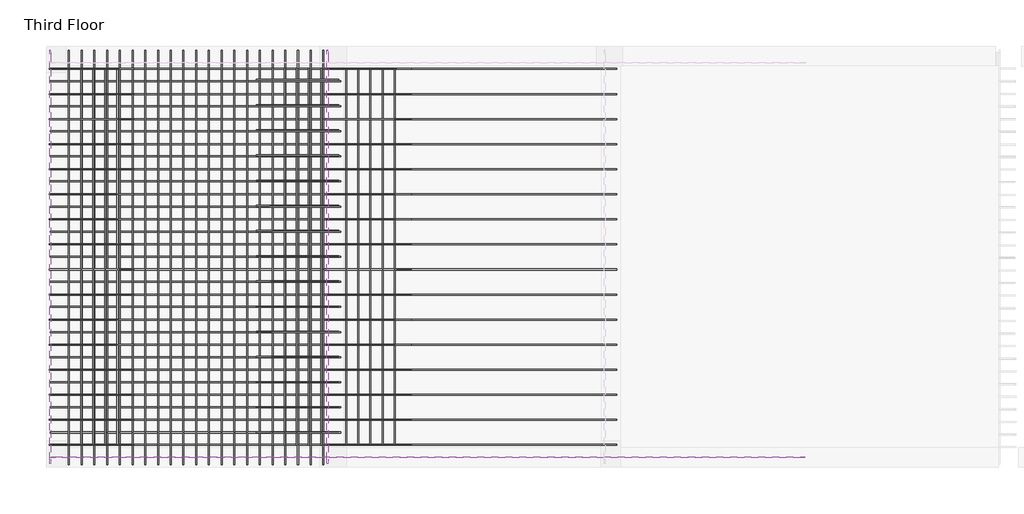
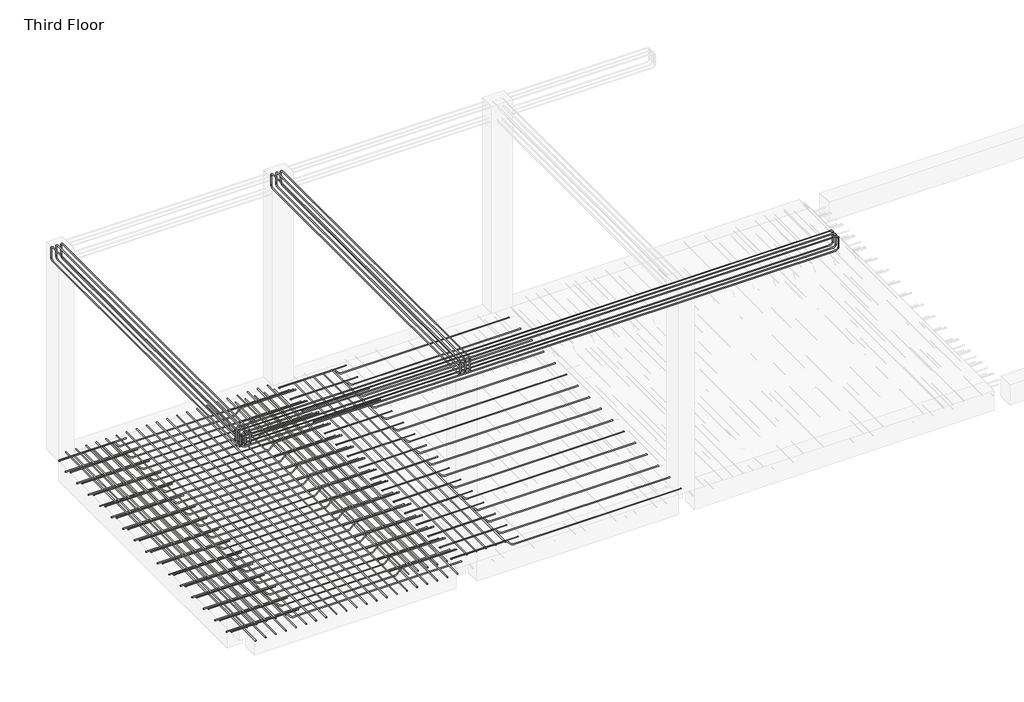
# One storey, part 2 of 4: 16 reinforcing bars.
"""IFC4 building model written with IfcOpenShell, lengths in millimetres."""

from ifc_helpers import new_model, si_unit, point, frame, origin, place, context, project, spatial, polyline, circle_curve, trimmed, segment, composite_curve, source, transform, mapped, element, save
from ifc_brep_helpers import swept_disk

model = new_model("IFC4")

# Units and contexts
model_context = context("Model", 3, world=origin())
ifc_project = project(units=[si_unit("LENGTHUNIT", "METRE", prefix="MILLI")], contexts=[model_context])

# Site, building, storey
site = spatial("IfcSite", under=ifc_project)
building = spatial("IfcBuilding", under=site)
storey = spatial("IfcBuildingStorey", under=building, Name="Third Floor", Elevation=9601.2)

# Reinforcing bars
placement = place(None, origin())
reinforcing_bar_shape = source(origin(), model_context, "Body", "SolidModel", [
    swept_disk(composite_curve([segment(polyline([(-9335.8112474, 5017.2334631, 12564.4994949), (-9335.8112474, 5017.2334631, 12712.4994949)]), True, "CONTINUOUS"), segment(trimmed(circle_curve(frame((-9335.8112474, 4971.2334631, 12712.4994949), z_axis=(1.0, 0.0, 0.0), x_axis=(0.0, 46.0, 0.0)), 46.0), [point((-9335.8112474, 5017.2334631, 12712.4994949))], [point((-9335.8112474, 4971.2334631, 12758.4994949))], True, "CARTESIAN"), True, "CONTINUOUS"), segment(polyline([(-9335.8112474, 4971.2334631, 12758.4994949), (-9335.8112474, 278.4334631, 12758.4994949)]), True, "CONTINUOUS"), segment(trimmed(circle_curve(frame((-9335.8112474, 278.4334631, 12712.4994949), z_axis=(1.0, 0.0, 0.0), x_axis=(0.0, 0.0, 46.0)), 46.0), [point((-9335.8112474, 278.4334631, 12758.4994949))], [point((-9335.8112474, 232.4334631, 12712.4994949))], True, "CARTESIAN"), True, "CONTINUOUS"), segment(polyline([(-9335.8112474, 232.4334631, 12712.4994949), (-9335.8112474, 232.4334631, 12564.4994949)]), True, "CONTINUOUS")], self_intersect=False), 6.0),
])
element("IfcReinforcingBar", 1, at=placement, inside=storey, context=model_context, shape_type="MappedRepresentation", body=[
    mapped(reinforcing_bar_shape, transform((0.0, 0.0, 0.0), x_axis=(1.0, 0.0, 0.0), y_axis=(0.0, 1.0, 0.0), z_axis=(0.0, 0.0, 1.0))),
    mapped(reinforcing_bar_shape, transform((71.1994949, 0.0, 0.0), x_axis=(1.0, 0.0, 0.0), y_axis=(0.0, 1.0, 0.0), z_axis=(0.0, 0.0, 1.0))),
    mapped(reinforcing_bar_shape, transform((142.3989899, 0.0, 0.0), x_axis=(1.0, 0.0, 0.0), y_axis=(0.0, 1.0, 0.0), z_axis=(0.0, 0.0, 1.0))),
])
reinforcing_bar_2_shape = source(origin(), model_context, "Body", "SolidModel", [
    swept_disk(composite_curve([segment(polyline([(-9335.8112474, 5017.2334631, 12733.9005051), (-9335.8112474, 5017.2334631, 12585.9005051)]), True, "CONTINUOUS"), segment(trimmed(circle_curve(frame((-9335.8112474, 4971.2334631, 12585.9005051), z_axis=(-1.0, 0.0, 0.0), x_axis=(0.0, 46.0, 0.0)), 46.0), [point((-9335.8112474, 5017.2334631, 12585.9005051))], [point((-9335.8112474, 4971.2334631, 12539.9005051))], True, "CARTESIAN"), True, "CONTINUOUS"), segment(polyline([(-9335.8112474, 4971.2334631, 12539.9005051), (-9335.8112474, 278.4334631, 12539.9005051)]), True, "CONTINUOUS"), segment(trimmed(circle_curve(frame((-9335.8112474, 278.4334631, 12585.9005051), z_axis=(-1.0, 0.0, 0.0), x_axis=(0.0, 0.0, -46.0)), 46.0), [point((-9335.8112474, 278.4334631, 12539.9005051))], [point((-9335.8112474, 232.4334631, 12585.9005051))], True, "CARTESIAN"), True, "CONTINUOUS"), segment(polyline([(-9335.8112474, 232.4334631, 12585.9005051), (-9335.8112474, 232.4334631, 12733.9005051)]), True, "CONTINUOUS")], self_intersect=False), 6.0),
])
element("IfcReinforcingBar", 2, at=placement, inside=storey, context=model_context, shape_type="MappedRepresentation", body=[
    mapped(reinforcing_bar_2_shape, transform((0.0, 0.0, 0.0), x_axis=(1.0, 0.0, 0.0), y_axis=(0.0, 1.0, 0.0), z_axis=(0.0, 0.0, 1.0))),
    mapped(reinforcing_bar_2_shape, transform((71.1994949, 0.0, 0.0), x_axis=(1.0, 0.0, 0.0), y_axis=(0.0, 1.0, 0.0), z_axis=(0.0, 0.0, 1.0))),
    mapped(reinforcing_bar_2_shape, transform((142.3989899, 0.0, 0.0), x_axis=(1.0, 0.0, 0.0), y_axis=(0.0, 1.0, 0.0), z_axis=(0.0, 0.0, 1.0))),
])
reinforcing_bar_3_shape = source(origin(), model_context, "Body", "SolidModel", [
    swept_disk(composite_curve([segment(polyline([(-6122.7112474, 5017.2334631, 12564.4994949), (-6122.7112474, 5017.2334631, 12712.4994949)]), True, "CONTINUOUS"), segment(trimmed(circle_curve(frame((-6122.7112474, 4971.2334631, 12712.4994949), z_axis=(1.0, 0.0, 0.0), x_axis=(0.0, 46.0, 0.0)), 46.0), [point((-6122.7112474, 5017.2334631, 12712.4994949))], [point((-6122.7112474, 4971.2334631, 12758.4994949))], True, "CARTESIAN"), True, "CONTINUOUS"), segment(polyline([(-6122.7112474, 4971.2334631, 12758.4994949), (-6122.7112474, 278.4334631, 12758.4994949)]), True, "CONTINUOUS"), segment(trimmed(circle_curve(frame((-6122.7112474, 278.4334631, 12712.4994949), z_axis=(1.0, 0.0, 0.0), x_axis=(0.0, 0.0, 46.0)), 46.0), [point((-6122.7112474, 278.4334631, 12758.4994949))], [point((-6122.7112474, 232.4334631, 12712.4994949))], True, "CARTESIAN"), True, "CONTINUOUS"), segment(polyline([(-6122.7112474, 232.4334631, 12712.4994949), (-6122.7112474, 232.4334631, 12564.4994949)]), True, "CONTINUOUS")], self_intersect=False), 6.0),
])
element("IfcReinforcingBar", 3, at=placement, inside=storey, context=model_context, shape_type="MappedRepresentation", body=[
    mapped(reinforcing_bar_3_shape, transform((0.0, 0.0, 0.0), x_axis=(1.0, 0.0, 0.0), y_axis=(0.0, 1.0, 0.0), z_axis=(0.0, 0.0, 1.0))),
    mapped(reinforcing_bar_3_shape, transform((71.1994949, 0.0, 0.0), x_axis=(1.0, 0.0, 0.0), y_axis=(0.0, 1.0, 0.0), z_axis=(0.0, 0.0, 1.0))),
    mapped(reinforcing_bar_3_shape, transform((142.3989899, 0.0, 0.0), x_axis=(1.0, 0.0, 0.0), y_axis=(0.0, 1.0, 0.0), z_axis=(0.0, 0.0, 1.0))),
])
reinforcing_bar_4_shape = source(origin(), model_context, "Body", "SolidModel", [
    swept_disk(composite_curve([segment(polyline([(-6122.7112474, 5017.2334631, 12733.9005051), (-6122.7112474, 5017.2334631, 12585.9005051)]), True, "CONTINUOUS"), segment(trimmed(circle_curve(frame((-6122.7112474, 4971.2334631, 12585.9005051), z_axis=(-1.0, 0.0, 0.0), x_axis=(0.0, 46.0, 0.0)), 46.0), [point((-6122.7112474, 5017.2334631, 12585.9005051))], [point((-6122.7112474, 4971.2334631, 12539.9005051))], True, "CARTESIAN"), True, "CONTINUOUS"), segment(polyline([(-6122.7112474, 4971.2334631, 12539.9005051), (-6122.7112474, 278.4334631, 12539.9005051)]), True, "CONTINUOUS"), segment(trimmed(circle_curve(frame((-6122.7112474, 278.4334631, 12585.9005051), z_axis=(-1.0, 0.0, 0.0), x_axis=(0.0, 0.0, -46.0)), 46.0), [point((-6122.7112474, 278.4334631, 12539.9005051))], [point((-6122.7112474, 232.4334631, 12585.9005051))], True, "CARTESIAN"), True, "CONTINUOUS"), segment(polyline([(-6122.7112474, 232.4334631, 12585.9005051), (-6122.7112474, 232.4334631, 12733.9005051)]), True, "CONTINUOUS")], self_intersect=False), 6.0),
])
element("IfcReinforcingBar", 4, at=placement, inside=storey, context=model_context, shape_type="MappedRepresentation", body=[
    mapped(reinforcing_bar_4_shape, transform((0.0, 0.0, 0.0), x_axis=(1.0, 0.0, 0.0), y_axis=(0.0, 1.0, 0.0), z_axis=(0.0, 0.0, 1.0))),
    mapped(reinforcing_bar_4_shape, transform((71.1994949, 0.0, 0.0), x_axis=(1.0, 0.0, 0.0), y_axis=(0.0, 1.0, 0.0), z_axis=(0.0, 0.0, 1.0))),
    mapped(reinforcing_bar_4_shape, transform((142.3989899, 0.0, 0.0), x_axis=(1.0, 0.0, 0.0), y_axis=(0.0, 1.0, 0.0), z_axis=(0.0, 0.0, 1.0))),
])
reinforcing_bar_5_shape = source(origin(), model_context, "Body", "SolidModel", [
    swept_disk(composite_curve([segment(polyline([(-9323.7564088, 229.5339681, 12564.4994949), (-9323.7564088, 229.5339681, 12712.4994949)]), True, "CONTINUOUS"), segment(trimmed(circle_curve(frame((-9277.7564088, 229.5339681, 12712.4994949), z_axis=(0.0, 1.0, 0.0), x_axis=(-46.0, 0.0, 0.0)), 46.0), [point((-9323.7564088, 229.5339681, 12712.4994949))], [point((-9277.7564088, 229.5339681, 12758.4994949))], True, "CARTESIAN"), True, "CONTINUOUS"), segment(polyline([(-9277.7564088, 229.5339681, 12758.4994949), (-642.1117524, 229.5339681, 12758.4994949)]), True, "CONTINUOUS"), segment(trimmed(circle_curve(frame((-642.1117524, 229.5339681, 12712.4994949), z_axis=(0.0, 1.0, 0.0), x_axis=(0.0, 0.0, 46.0)), 46.0), [point((-642.1117524, 229.5339681, 12758.4994949))], [point((-596.1117524, 229.5339681, 12712.4994949))], True, "CARTESIAN"), True, "CONTINUOUS"), segment(polyline([(-596.1117524, 229.5339681, 12712.4994949), (-596.1117524, 229.5339681, 12564.4994949)]), True, "CONTINUOUS")], self_intersect=False), 6.0),
])
element("IfcReinforcingBar", 5, at=placement, inside=storey, context=model_context, shape_type="MappedRepresentation", body=[
    mapped(reinforcing_bar_5_shape, transform((0.0, 0.0, 0.0), x_axis=(1.0, 0.0, 0.0), y_axis=(0.0, 1.0, 0.0), z_axis=(0.0, 0.0, 1.0))),
    mapped(reinforcing_bar_5_shape, transform((0.0, 71.1994949, 0.0), x_axis=(1.0, 0.0, 0.0), y_axis=(0.0, 1.0, 0.0), z_axis=(0.0, 0.0, 1.0))),
    mapped(reinforcing_bar_5_shape, transform((0.0, 142.3989899, 0.0), x_axis=(1.0, 0.0, 0.0), y_axis=(0.0, 1.0, 0.0), z_axis=(0.0, 0.0, 1.0))),
])
reinforcing_bar_6_shape = source(origin(), model_context, "Body", "SolidModel", [
    swept_disk(composite_curve([segment(polyline([(-9317.575971, 229.5339681, 12733.9005051), (-9317.575971, 229.5339681, 12585.9005051)]), True, "CONTINUOUS"), segment(trimmed(circle_curve(frame((-9271.575971, 229.5339681, 12585.9005051), z_axis=(0.0, -1.0, 0.0), x_axis=(-46.0, 0.0, 0.0)), 46.0), [point((-9317.575971, 229.5339681, 12585.9005051))], [point((-9271.575971, 229.5339681, 12539.9005051))], True, "CARTESIAN"), True, "CONTINUOUS"), segment(polyline([(-9271.575971, 229.5339681, 12539.9005051), (-642.1117524, 229.5339681, 12539.9005051)]), True, "CONTINUOUS"), segment(trimmed(circle_curve(frame((-642.1117524, 229.5339681, 12585.9005051), z_axis=(0.0, -1.0, 0.0), x_axis=(0.0, 0.0, -46.0)), 46.0), [point((-642.1117524, 229.5339681, 12539.9005051))], [point((-596.1117524, 229.5339681, 12585.9005051))], True, "CARTESIAN"), True, "CONTINUOUS"), segment(polyline([(-596.1117524, 229.5339681, 12585.9005051), (-596.1117524, 229.5339681, 12733.9005051)]), True, "CONTINUOUS")], self_intersect=False), 6.0),
])
element("IfcReinforcingBar", 6, at=placement, inside=storey, context=model_context, shape_type="MappedRepresentation", body=[
    mapped(reinforcing_bar_6_shape, transform((0.0, 0.0, 0.0), x_axis=(1.0, 0.0, 0.0), y_axis=(0.0, 1.0, 0.0), z_axis=(0.0, 0.0, 1.0))),
    mapped(reinforcing_bar_6_shape, transform((0.0, 71.1994949, 0.0), x_axis=(1.0, 0.0, 0.0), y_axis=(0.0, 1.0, 0.0), z_axis=(0.0, 0.0, 1.0))),
    mapped(reinforcing_bar_6_shape, transform((0.0, 142.3989899, 0.0), x_axis=(1.0, 0.0, 0.0), y_axis=(0.0, 1.0, 0.0), z_axis=(0.0, 0.0, 1.0))),
])
reinforcing_bar_7_shape = source(origin(), model_context, "Body", "SolidModel", [
    swept_disk(composite_curve([segment(polyline([(-9347.5125695, 4803.6334631, 9570.2), (-8565.5792829, 4803.6334631, 9570.2)]), True, "CONTINUOUS"), segment(trimmed(circle_curve(frame((-8565.5792829, 4803.6334631, 9524.2), z_axis=(0.0, 1.0, 0.0), x_axis=(0.0, 0.0, 46.0)), 46.0), [point((-8565.5792829, 4803.6334631, 9570.2))], [point((-8533.052371, 4803.6334631, 9556.7269119))], True, "CARTESIAN"), True, "CONTINUOUS"), segment(polyline([(-8533.052371, 4803.6334631, 9556.7269119), (-8469.5985471, 4803.6334631, 9493.2730881)]), True, "CONTINUOUS"), segment(trimmed(circle_curve(frame((-8437.0716352, 4803.6334631, 9525.8), z_axis=(0.0, -1.0000000000000002, 0.0), x_axis=(-32.526911900000414, 0.0, -32.526911899998595)), 46.0), [point((-8469.5985471, 4803.6334631, 9493.2730881))], [point((-8437.0716352, 4803.6334631, 9479.8))], True, "CARTESIAN"), True, "CONTINUOUS"), segment(polyline([(-8437.0716352, 4803.6334631, 9479.8), (-5982.0597449, 4803.6334631, 9479.8)]), True, "CONTINUOUS")], self_intersect=False), 6.0),
])
element("IfcReinforcingBar", 7, at=placement, inside=storey, context=model_context, shape_type="MappedRepresentation", body=[
    mapped(reinforcing_bar_7_shape, transform((0.0, 0.0, 0.0), x_axis=(1.0, 0.0, 0.0), y_axis=(0.0, 1.0, 0.0), z_axis=(0.0, 0.0, 1.0))),
    mapped(reinforcing_bar_7_shape, transform((0.0, -290.5066667, 0.0), x_axis=(1.0, 0.0, 0.0), y_axis=(0.0, 1.0, 0.0), z_axis=(0.0, 0.0, 1.0))),
    mapped(reinforcing_bar_7_shape, transform((0.0, -581.0133333, 0.0), x_axis=(1.0, 0.0, 0.0), y_axis=(0.0, 1.0, 0.0), z_axis=(0.0, 0.0, 1.0))),
    mapped(reinforcing_bar_7_shape, transform((0.0, -871.52, 0.0), x_axis=(1.0, 0.0, 0.0), y_axis=(0.0, 1.0, 0.0), z_axis=(0.0, 0.0, 1.0))),
    mapped(reinforcing_bar_7_shape, transform((0.0, -1162.0266667, 0.0), x_axis=(1.0, 0.0, 0.0), y_axis=(0.0, 1.0, 0.0), z_axis=(0.0, 0.0, 1.0))),
    mapped(reinforcing_bar_7_shape, transform((0.0, -1452.5333333, 0.0), x_axis=(1.0, 0.0, 0.0), y_axis=(0.0, 1.0, 0.0), z_axis=(0.0, 0.0, 1.0))),
    mapped(reinforcing_bar_7_shape, transform((0.0, -1743.04, 0.0), x_axis=(1.0, 0.0, 0.0), y_axis=(0.0, 1.0, 0.0), z_axis=(0.0, 0.0, 1.0))),
    mapped(reinforcing_bar_7_shape, transform((0.0, -2033.5466667, 0.0), x_axis=(1.0, 0.0, 0.0), y_axis=(0.0, 1.0, 0.0), z_axis=(0.0, 0.0, 1.0))),
    mapped(reinforcing_bar_7_shape, transform((0.0, -2324.0533333, 0.0), x_axis=(1.0, 0.0, 0.0), y_axis=(0.0, 1.0, 0.0), z_axis=(0.0, 0.0, 1.0))),
    mapped(reinforcing_bar_7_shape, transform((0.0, -2614.56, 0.0), x_axis=(1.0, 0.0, 0.0), y_axis=(0.0, 1.0, 0.0), z_axis=(0.0, 0.0, 1.0))),
    mapped(reinforcing_bar_7_shape, transform((0.0, -2905.0666667, 0.0), x_axis=(1.0, 0.0, 0.0), y_axis=(0.0, 1.0, 0.0), z_axis=(0.0, 0.0, 1.0))),
    mapped(reinforcing_bar_7_shape, transform((0.0, -3195.5733333, 0.0), x_axis=(1.0, 0.0, 0.0), y_axis=(0.0, 1.0, 0.0), z_axis=(0.0, 0.0, 1.0))),
    mapped(reinforcing_bar_7_shape, transform((0.0, -3486.08, 0.0), x_axis=(1.0, 0.0, 0.0), y_axis=(0.0, 1.0, 0.0), z_axis=(0.0, 0.0, 1.0))),
    mapped(reinforcing_bar_7_shape, transform((0.0, -3776.5866667, 0.0), x_axis=(1.0, 0.0, 0.0), y_axis=(0.0, 1.0, 0.0), z_axis=(0.0, 0.0, 1.0))),
    mapped(reinforcing_bar_7_shape, transform((0.0, -4067.0933333, 0.0), x_axis=(1.0, 0.0, 0.0), y_axis=(0.0, 1.0, 0.0), z_axis=(0.0, 0.0, 1.0))),
    mapped(reinforcing_bar_7_shape, transform((0.0, -4357.6, 0.0), x_axis=(1.0, 0.0, 0.0), y_axis=(0.0, 1.0, 0.0), z_axis=(0.0, 0.0, 1.0))),
])
reinforcing_bar_8_shape = source(origin(), model_context, "Body", "SolidModel", [
    swept_disk(composite_curve([segment(polyline([(-5968.6109354, 590.4513536, 9570.2), (-6750.544222, 590.4513536, 9570.2)]), True, "CONTINUOUS"), segment(trimmed(circle_curve(frame((-6750.544222, 590.4513536, 9524.2), z_axis=(0.0, -1.0, 0.0), x_axis=(0.0, 0.0, 46.0)), 46.0), [point((-6750.544222, 590.4513536, 9570.2))], [point((-6783.0711339, 590.4513536, 9556.7269119))], True, "CARTESIAN"), True, "CONTINUOUS"), segment(polyline([(-6783.0711339, 590.4513536, 9556.7269119), (-6846.5249578, 590.4513536, 9493.2730881)]), True, "CONTINUOUS"), segment(trimmed(circle_curve(frame((-6879.0518697, 590.4513536, 9525.8), z_axis=(0.0, 1.0000000000000002, 0.0), x_axis=(32.526911899999504, 0.0, -32.526911899998595)), 46.0), [point((-6846.5249578, 590.4513536, 9493.2730881))], [point((-6879.0518697, 590.4513536, 9479.8))], True, "CARTESIAN"), True, "CONTINUOUS"), segment(polyline([(-6879.0518697, 590.4513536, 9479.8), (-9334.06376, 590.4513536, 9479.8)]), True, "CONTINUOUS")], self_intersect=False), 6.0),
])
element("IfcReinforcingBar", 8, at=placement, inside=storey, context=model_context, shape_type="MappedRepresentation", body=[
    mapped(reinforcing_bar_8_shape, transform((0.0, 0.0, 0.0), x_axis=(1.0, 0.0, 0.0), y_axis=(0.0, 1.0, 0.0), z_axis=(0.0, 0.0, 1.0))),
    mapped(reinforcing_bar_8_shape, transform((0.0, 290.9296088, 0.0), x_axis=(1.0, 0.0, 0.0), y_axis=(0.0, 1.0, 0.0), z_axis=(0.0, 0.0, 1.0))),
    mapped(reinforcing_bar_8_shape, transform((0.0, 581.8592177, 0.0), x_axis=(1.0, 0.0, 0.0), y_axis=(0.0, 1.0, 0.0), z_axis=(0.0, 0.0, 1.0))),
    mapped(reinforcing_bar_8_shape, transform((0.0, 872.7888265, 0.0), x_axis=(1.0, 0.0, 0.0), y_axis=(0.0, 1.0, 0.0), z_axis=(0.0, 0.0, 1.0))),
    mapped(reinforcing_bar_8_shape, transform((0.0, 1163.7184353, 0.0), x_axis=(1.0, 0.0, 0.0), y_axis=(0.0, 1.0, 0.0), z_axis=(0.0, 0.0, 1.0))),
    mapped(reinforcing_bar_8_shape, transform((0.0, 1454.6480442, 0.0), x_axis=(1.0, 0.0, 0.0), y_axis=(0.0, 1.0, 0.0), z_axis=(0.0, 0.0, 1.0))),
    mapped(reinforcing_bar_8_shape, transform((0.0, 1745.577653, 0.0), x_axis=(1.0, 0.0, 0.0), y_axis=(0.0, 1.0, 0.0), z_axis=(0.0, 0.0, 1.0))),
    mapped(reinforcing_bar_8_shape, transform((0.0, 2036.5072618, 0.0), x_axis=(1.0, 0.0, 0.0), y_axis=(0.0, 1.0, 0.0), z_axis=(0.0, 0.0, 1.0))),
    mapped(reinforcing_bar_8_shape, transform((0.0, 2327.4368707, 0.0), x_axis=(1.0, 0.0, 0.0), y_axis=(0.0, 1.0, 0.0), z_axis=(0.0, 0.0, 1.0))),
    mapped(reinforcing_bar_8_shape, transform((0.0, 2618.3664795, 0.0), x_axis=(1.0, 0.0, 0.0), y_axis=(0.0, 1.0, 0.0), z_axis=(0.0, 0.0, 1.0))),
    mapped(reinforcing_bar_8_shape, transform((0.0, 2909.2960883, 0.0), x_axis=(1.0, 0.0, 0.0), y_axis=(0.0, 1.0, 0.0), z_axis=(0.0, 0.0, 1.0))),
    mapped(reinforcing_bar_8_shape, transform((0.0, 3200.2256972, 0.0), x_axis=(1.0, 0.0, 0.0), y_axis=(0.0, 1.0, 0.0), z_axis=(0.0, 0.0, 1.0))),
    mapped(reinforcing_bar_8_shape, transform((0.0, 3491.155306, 0.0), x_axis=(1.0, 0.0, 0.0), y_axis=(0.0, 1.0, 0.0), z_axis=(0.0, 0.0, 1.0))),
    mapped(reinforcing_bar_8_shape, transform((0.0, 3782.0849148, 0.0), x_axis=(1.0, 0.0, 0.0), y_axis=(0.0, 1.0, 0.0), z_axis=(0.0, 0.0, 1.0))),
    mapped(reinforcing_bar_8_shape, transform((0.0, 4073.0145236, 0.0), x_axis=(1.0, 0.0, 0.0), y_axis=(0.0, 1.0, 0.0), z_axis=(0.0, 0.0, 1.0))),
])
reinforcing_bar_9_shape = source(origin(), model_context, "Body", "SolidModel", [
    swept_disk(composite_curve([segment(polyline([(-8556.5984173, 4809.6334631, 9559.9006995), (-8556.5984173, 440.0334631, 9559.9006995)]), True, "CONTINUOUS")], self_intersect=False), 6.0),
])
element("IfcReinforcingBar", 9, at=placement, inside=storey, context=model_context, shape_type="MappedRepresentation", body=[
    mapped(reinforcing_bar_9_shape, transform((0.0, 0.0, 0.0), x_axis=(1.0, 0.0, 0.0), y_axis=(0.0, 1.0, 0.0), z_axis=(0.0, 0.0, 1.0))),
    mapped(reinforcing_bar_9_shape, transform((-140.6783338, 0.0, 0.0), x_axis=(1.0, 0.0, 0.0), y_axis=(0.0, 1.0, 0.0), z_axis=(0.0, 0.0, 1.0))),
    mapped(reinforcing_bar_9_shape, transform((-281.3566676, 0.0, 0.0), x_axis=(1.0, 0.0, 0.0), y_axis=(0.0, 1.0, 0.0), z_axis=(0.0, 0.0, 1.0))),
    mapped(reinforcing_bar_9_shape, transform((-422.0350014, 0.0, 0.0), x_axis=(1.0, 0.0, 0.0), y_axis=(0.0, 1.0, 0.0), z_axis=(0.0, 0.0, 1.0))),
    mapped(reinforcing_bar_9_shape, transform((-562.7133352, 0.0, 0.0), x_axis=(1.0, 0.0, 0.0), y_axis=(0.0, 1.0, 0.0), z_axis=(0.0, 0.0, 1.0))),
])
reinforcing_bar_10_shape = source(origin(), model_context, "Body", "SolidModel", [
    swept_disk(composite_curve([segment(polyline([(-6759.5250876, 4809.6334631, 9559.9006995), (-6759.5250876, 440.0334631, 9559.9006995)]), True, "CONTINUOUS")], self_intersect=False), 6.0),
])
element("IfcReinforcingBar", 10, at=placement, inside=storey, context=model_context, shape_type="MappedRepresentation", body=[
    mapped(reinforcing_bar_10_shape, transform((0.0, 0.0, 0.0), x_axis=(1.0, 0.0, 0.0), y_axis=(0.0, 1.0, 0.0), z_axis=(0.0, 0.0, 1.0))),
    mapped(reinforcing_bar_10_shape, transform((140.6783338, 0.0, 0.0), x_axis=(1.0, 0.0, 0.0), y_axis=(0.0, 1.0, 0.0), z_axis=(0.0, 0.0, 1.0))),
    mapped(reinforcing_bar_10_shape, transform((281.3566676, 0.0, 0.0), x_axis=(1.0, 0.0, 0.0), y_axis=(0.0, 1.0, 0.0), z_axis=(0.0, 0.0, 1.0))),
    mapped(reinforcing_bar_10_shape, transform((422.0350014, 0.0, 0.0), x_axis=(1.0, 0.0, 0.0), y_axis=(0.0, 1.0, 0.0), z_axis=(0.0, 0.0, 1.0))),
    mapped(reinforcing_bar_10_shape, transform((562.7133352, 0.0, 0.0), x_axis=(1.0, 0.0, 0.0), y_axis=(0.0, 1.0, 0.0), z_axis=(0.0, 0.0, 1.0))),
])
reinforcing_bar_11_shape = source(origin(), model_context, "Body", "SolidModel", [
    swept_disk(composite_curve([segment(polyline([(-9338.4522926, 4805.6334631, 9572.2), (-8365.7369752, 4805.6334631, 9572.2)]), True, "CONTINUOUS")], self_intersect=False), 4.0),
])
element("IfcReinforcingBar", 11, at=placement, inside=storey, context=model_context, shape_type="MappedRepresentation", body=[
    mapped(reinforcing_bar_11_shape, transform((0.0, 0.0, 0.0), x_axis=(1.0, 0.0, 0.0), y_axis=(0.0, 1.0, 0.0), z_axis=(0.0, 0.0, 1.0))),
    mapped(reinforcing_bar_11_shape, transform((0.0, -290.7733333, 0.0), x_axis=(1.0, 0.0, 0.0), y_axis=(0.0, 1.0, 0.0), z_axis=(0.0, 0.0, 1.0))),
    mapped(reinforcing_bar_11_shape, transform((0.0, -581.5466667, 0.0), x_axis=(1.0, 0.0, 0.0), y_axis=(0.0, 1.0, 0.0), z_axis=(0.0, 0.0, 1.0))),
    mapped(reinforcing_bar_11_shape, transform((0.0, -872.32, 0.0), x_axis=(1.0, 0.0, 0.0), y_axis=(0.0, 1.0, 0.0), z_axis=(0.0, 0.0, 1.0))),
    mapped(reinforcing_bar_11_shape, transform((0.0, -1163.0933333, 0.0), x_axis=(1.0, 0.0, 0.0), y_axis=(0.0, 1.0, 0.0), z_axis=(0.0, 0.0, 1.0))),
    mapped(reinforcing_bar_11_shape, transform((0.0, -1453.8666667, 0.0), x_axis=(1.0, 0.0, 0.0), y_axis=(0.0, 1.0, 0.0), z_axis=(0.0, 0.0, 1.0))),
    mapped(reinforcing_bar_11_shape, transform((0.0, -1744.64, 0.0), x_axis=(1.0, 0.0, 0.0), y_axis=(0.0, 1.0, 0.0), z_axis=(0.0, 0.0, 1.0))),
    mapped(reinforcing_bar_11_shape, transform((0.0, -2035.4133333, 0.0), x_axis=(1.0, 0.0, 0.0), y_axis=(0.0, 1.0, 0.0), z_axis=(0.0, 0.0, 1.0))),
    mapped(reinforcing_bar_11_shape, transform((0.0, -2326.1866667, 0.0), x_axis=(1.0, 0.0, 0.0), y_axis=(0.0, 1.0, 0.0), z_axis=(0.0, 0.0, 1.0))),
    mapped(reinforcing_bar_11_shape, transform((0.0, -2616.96, 0.0), x_axis=(1.0, 0.0, 0.0), y_axis=(0.0, 1.0, 0.0), z_axis=(0.0, 0.0, 1.0))),
    mapped(reinforcing_bar_11_shape, transform((0.0, -2907.7333333, 0.0), x_axis=(1.0, 0.0, 0.0), y_axis=(0.0, 1.0, 0.0), z_axis=(0.0, 0.0, 1.0))),
    mapped(reinforcing_bar_11_shape, transform((0.0, -3198.5066667, 0.0), x_axis=(1.0, 0.0, 0.0), y_axis=(0.0, 1.0, 0.0), z_axis=(0.0, 0.0, 1.0))),
    mapped(reinforcing_bar_11_shape, transform((0.0, -3489.28, 0.0), x_axis=(1.0, 0.0, 0.0), y_axis=(0.0, 1.0, 0.0), z_axis=(0.0, 0.0, 1.0))),
    mapped(reinforcing_bar_11_shape, transform((0.0, -3780.0533333, 0.0), x_axis=(1.0, 0.0, 0.0), y_axis=(0.0, 1.0, 0.0), z_axis=(0.0, 0.0, 1.0))),
    mapped(reinforcing_bar_11_shape, transform((0.0, -4070.8266667, 0.0), x_axis=(1.0, 0.0, 0.0), y_axis=(0.0, 1.0, 0.0), z_axis=(0.0, 0.0, 1.0))),
    mapped(reinforcing_bar_11_shape, transform((0.0, -4361.6, 0.0), x_axis=(1.0, 0.0, 0.0), y_axis=(0.0, 1.0, 0.0), z_axis=(0.0, 0.0, 1.0))),
])
reinforcing_bar_12_shape = source(origin(), model_context, "Body", "SolidModel", [
    swept_disk(composite_curve([segment(polyline([(-5991.3123639, 4678.4115375, 9572.2), (-6950.3865297, 4678.4115375, 9572.2)]), True, "CONTINUOUS")], self_intersect=False), 4.0),
])
element("IfcReinforcingBar", 12, at=placement, inside=storey, context=model_context, shape_type="MappedRepresentation", body=[
    mapped(reinforcing_bar_12_shape, transform((0.0, 0.0, 0.0), x_axis=(1.0, 0.0, 0.0), y_axis=(0.0, 1.0, 0.0), z_axis=(0.0, 0.0, 1.0))),
    mapped(reinforcing_bar_12_shape, transform((0.0, -291.8025106, 0.0), x_axis=(1.0, 0.0, 0.0), y_axis=(0.0, 1.0, 0.0), z_axis=(0.0, 0.0, 1.0))),
    mapped(reinforcing_bar_12_shape, transform((0.0, -583.6050212, 0.0), x_axis=(1.0, 0.0, 0.0), y_axis=(0.0, 1.0, 0.0), z_axis=(0.0, 0.0, 1.0))),
    mapped(reinforcing_bar_12_shape, transform((0.0, -875.4075319, 0.0), x_axis=(1.0, 0.0, 0.0), y_axis=(0.0, 1.0, 0.0), z_axis=(0.0, 0.0, 1.0))),
    mapped(reinforcing_bar_12_shape, transform((0.0, -1167.2100425, 0.0), x_axis=(1.0, 0.0, 0.0), y_axis=(0.0, 1.0, 0.0), z_axis=(0.0, 0.0, 1.0))),
    mapped(reinforcing_bar_12_shape, transform((0.0, -1459.0125531, 0.0), x_axis=(1.0, 0.0, 0.0), y_axis=(0.0, 1.0, 0.0), z_axis=(0.0, 0.0, 1.0))),
    mapped(reinforcing_bar_12_shape, transform((0.0, -1750.8150637, 0.0), x_axis=(1.0, 0.0, 0.0), y_axis=(0.0, 1.0, 0.0), z_axis=(0.0, 0.0, 1.0))),
    mapped(reinforcing_bar_12_shape, transform((0.0, -2042.6175743, 0.0), x_axis=(1.0, 0.0, 0.0), y_axis=(0.0, 1.0, 0.0), z_axis=(0.0, 0.0, 1.0))),
    mapped(reinforcing_bar_12_shape, transform((0.0, -2334.420085, 0.0), x_axis=(1.0, 0.0, 0.0), y_axis=(0.0, 1.0, 0.0), z_axis=(0.0, 0.0, 1.0))),
    mapped(reinforcing_bar_12_shape, transform((0.0, -2626.2225956, 0.0), x_axis=(1.0, 0.0, 0.0), y_axis=(0.0, 1.0, 0.0), z_axis=(0.0, 0.0, 1.0))),
    mapped(reinforcing_bar_12_shape, transform((0.0, -2918.0251062, 0.0), x_axis=(1.0, 0.0, 0.0), y_axis=(0.0, 1.0, 0.0), z_axis=(0.0, 0.0, 1.0))),
    mapped(reinforcing_bar_12_shape, transform((0.0, -3209.8276168, 0.0), x_axis=(1.0, 0.0, 0.0), y_axis=(0.0, 1.0, 0.0), z_axis=(0.0, 0.0, 1.0))),
    mapped(reinforcing_bar_12_shape, transform((0.0, -3501.6301274, 0.0), x_axis=(1.0, 0.0, 0.0), y_axis=(0.0, 1.0, 0.0), z_axis=(0.0, 0.0, 1.0))),
    mapped(reinforcing_bar_12_shape, transform((0.0, -3793.4326381, 0.0), x_axis=(1.0, 0.0, 0.0), y_axis=(0.0, 1.0, 0.0), z_axis=(0.0, 0.0, 1.0))),
    mapped(reinforcing_bar_12_shape, transform((0.0, -4085.2351487, 0.0), x_axis=(1.0, 0.0, 0.0), y_axis=(0.0, 1.0, 0.0), z_axis=(0.0, 0.0, 1.0))),
])
reinforcing_bar_13_shape = source(origin(), model_context, "Body", "SolidModel", [
    swept_disk(composite_curve([segment(polyline([(-6169.8117524, 218.9117605, 9488.3387401), (-6169.8117524, 5019.9992064, 9488.3387401)]), True, "CONTINUOUS")], self_intersect=False), 6.0),
])
element("IfcReinforcingBar", 13, at=placement, inside=storey, context=model_context, shape_type="MappedRepresentation", body=[
    mapped(reinforcing_bar_13_shape, transform((0.0, 0.0, 0.0), x_axis=(1.0, 0.0, 0.0), y_axis=(0.0, 1.0, 0.0), z_axis=(0.0, 0.0, 1.0))),
    mapped(reinforcing_bar_13_shape, transform((-147.475, 0.0, 0.0), x_axis=(1.0, 0.0, 0.0), y_axis=(0.0, 1.0, 0.0), z_axis=(0.0, 0.0, 1.0))),
    mapped(reinforcing_bar_13_shape, transform((-294.95, 0.0, 0.0), x_axis=(1.0, 0.0, 0.0), y_axis=(0.0, 1.0, 0.0), z_axis=(0.0, 0.0, 1.0))),
    mapped(reinforcing_bar_13_shape, transform((-442.425, 0.0, 0.0), x_axis=(1.0, 0.0, 0.0), y_axis=(0.0, 1.0, 0.0), z_axis=(0.0, 0.0, 1.0))),
    mapped(reinforcing_bar_13_shape, transform((-589.9, 0.0, 0.0), x_axis=(1.0, 0.0, 0.0), y_axis=(0.0, 1.0, 0.0), z_axis=(0.0, 0.0, 1.0))),
    mapped(reinforcing_bar_13_shape, transform((-737.375, 0.0, 0.0), x_axis=(1.0, 0.0, 0.0), y_axis=(0.0, 1.0, 0.0), z_axis=(0.0, 0.0, 1.0))),
    mapped(reinforcing_bar_13_shape, transform((-884.85, 0.0, 0.0), x_axis=(1.0, 0.0, 0.0), y_axis=(0.0, 1.0, 0.0), z_axis=(0.0, 0.0, 1.0))),
    mapped(reinforcing_bar_13_shape, transform((-1032.325, 0.0, 0.0), x_axis=(1.0, 0.0, 0.0), y_axis=(0.0, 1.0, 0.0), z_axis=(0.0, 0.0, 1.0))),
    mapped(reinforcing_bar_13_shape, transform((-1179.8, 0.0, 0.0), x_axis=(1.0, 0.0, 0.0), y_axis=(0.0, 1.0, 0.0), z_axis=(0.0, 0.0, 1.0))),
    mapped(reinforcing_bar_13_shape, transform((-1327.275, 0.0, 0.0), x_axis=(1.0, 0.0, 0.0), y_axis=(0.0, 1.0, 0.0), z_axis=(0.0, 0.0, 1.0))),
    mapped(reinforcing_bar_13_shape, transform((-1474.75, 0.0, 0.0), x_axis=(1.0, 0.0, 0.0), y_axis=(0.0, 1.0, 0.0), z_axis=(0.0, 0.0, 1.0))),
    mapped(reinforcing_bar_13_shape, transform((-1622.225, 0.0, 0.0), x_axis=(1.0, 0.0, 0.0), y_axis=(0.0, 1.0, 0.0), z_axis=(0.0, 0.0, 1.0))),
    mapped(reinforcing_bar_13_shape, transform((-1769.7, 0.0, 0.0), x_axis=(1.0, 0.0, 0.0), y_axis=(0.0, 1.0, 0.0), z_axis=(0.0, 0.0, 1.0))),
    mapped(reinforcing_bar_13_shape, transform((-1917.175, 0.0, 0.0), x_axis=(1.0, 0.0, 0.0), y_axis=(0.0, 1.0, 0.0), z_axis=(0.0, 0.0, 1.0))),
    mapped(reinforcing_bar_13_shape, transform((-2064.65, 0.0, 0.0), x_axis=(1.0, 0.0, 0.0), y_axis=(0.0, 1.0, 0.0), z_axis=(0.0, 0.0, 1.0))),
    mapped(reinforcing_bar_13_shape, transform((-2212.125, 0.0, 0.0), x_axis=(1.0, 0.0, 0.0), y_axis=(0.0, 1.0, 0.0), z_axis=(0.0, 0.0, 1.0))),
    mapped(reinforcing_bar_13_shape, transform((-2359.6, 0.0, 0.0), x_axis=(1.0, 0.0, 0.0), y_axis=(0.0, 1.0, 0.0), z_axis=(0.0, 0.0, 1.0))),
    mapped(reinforcing_bar_13_shape, transform((-2507.075, 0.0, 0.0), x_axis=(1.0, 0.0, 0.0), y_axis=(0.0, 1.0, 0.0), z_axis=(0.0, 0.0, 1.0))),
    mapped(reinforcing_bar_13_shape, transform((-2654.55, 0.0, 0.0), x_axis=(1.0, 0.0, 0.0), y_axis=(0.0, 1.0, 0.0), z_axis=(0.0, 0.0, 1.0))),
    mapped(reinforcing_bar_13_shape, transform((-2802.025, 0.0, 0.0), x_axis=(1.0, 0.0, 0.0), y_axis=(0.0, 1.0, 0.0), z_axis=(0.0, 0.0, 1.0))),
    mapped(reinforcing_bar_13_shape, transform((-2949.5, 0.0, 0.0), x_axis=(1.0, 0.0, 0.0), y_axis=(0.0, 1.0, 0.0), z_axis=(0.0, 0.0, 1.0))),
])
reinforcing_bar_14_shape = source(origin(), model_context, "Body", "SolidModel", [
    swept_disk(composite_curve([segment(polyline([(-6134.4125695, 4803.6334631, 9570.2), (-5352.4792829, 4803.6334631, 9570.2)]), True, "CONTINUOUS"), segment(trimmed(circle_curve(frame((-5352.4792829, 4803.6334631, 9524.2), z_axis=(0.0, 1.0, 0.0), x_axis=(0.0, 0.0, 46.0)), 46.0), [point((-5352.4792829, 4803.6334631, 9570.2))], [point((-5319.952371, 4803.6334631, 9556.7269119))], True, "CARTESIAN"), True, "CONTINUOUS"), segment(polyline([(-5319.952371, 4803.6334631, 9556.7269119), (-5256.4985471, 4803.6334631, 9493.2730881)]), True, "CONTINUOUS"), segment(trimmed(circle_curve(frame((-5223.9716352, 4803.6334631, 9525.8), z_axis=(0.0, -1.0000000000000002, 0.0), x_axis=(-32.526911900000414, 0.0, -32.526911899998595)), 46.0), [point((-5256.4985471, 4803.6334631, 9493.2730881))], [point((-5223.9716352, 4803.6334631, 9479.8))], True, "CARTESIAN"), True, "CONTINUOUS"), segment(polyline([(-5223.9716352, 4803.6334631, 9479.8), (-2768.9597449, 4803.6334631, 9479.8)]), True, "CONTINUOUS")], self_intersect=False), 6.0),
])
element("IfcReinforcingBar", 14, at=placement, inside=storey, context=model_context, shape_type="MappedRepresentation", body=[
    mapped(reinforcing_bar_14_shape, transform((0.0, 0.0, 0.0), x_axis=(1.0, 0.0, 0.0), y_axis=(0.0, 1.0, 0.0), z_axis=(0.0, 0.0, 1.0))),
    mapped(reinforcing_bar_14_shape, transform((0.0, -290.5066667, 0.0), x_axis=(1.0, 0.0, 0.0), y_axis=(0.0, 1.0, 0.0), z_axis=(0.0, 0.0, 1.0))),
    mapped(reinforcing_bar_14_shape, transform((0.0, -581.0133333, 0.0), x_axis=(1.0, 0.0, 0.0), y_axis=(0.0, 1.0, 0.0), z_axis=(0.0, 0.0, 1.0))),
    mapped(reinforcing_bar_14_shape, transform((0.0, -871.52, 0.0), x_axis=(1.0, 0.0, 0.0), y_axis=(0.0, 1.0, 0.0), z_axis=(0.0, 0.0, 1.0))),
    mapped(reinforcing_bar_14_shape, transform((0.0, -1162.0266667, 0.0), x_axis=(1.0, 0.0, 0.0), y_axis=(0.0, 1.0, 0.0), z_axis=(0.0, 0.0, 1.0))),
    mapped(reinforcing_bar_14_shape, transform((0.0, -1452.5333333, 0.0), x_axis=(1.0, 0.0, 0.0), y_axis=(0.0, 1.0, 0.0), z_axis=(0.0, 0.0, 1.0))),
    mapped(reinforcing_bar_14_shape, transform((0.0, -1743.04, 0.0), x_axis=(1.0, 0.0, 0.0), y_axis=(0.0, 1.0, 0.0), z_axis=(0.0, 0.0, 1.0))),
    mapped(reinforcing_bar_14_shape, transform((0.0, -2033.5466667, 0.0), x_axis=(1.0, 0.0, 0.0), y_axis=(0.0, 1.0, 0.0), z_axis=(0.0, 0.0, 1.0))),
    mapped(reinforcing_bar_14_shape, transform((0.0, -2324.0533333, 0.0), x_axis=(1.0, 0.0, 0.0), y_axis=(0.0, 1.0, 0.0), z_axis=(0.0, 0.0, 1.0))),
    mapped(reinforcing_bar_14_shape, transform((0.0, -2614.56, 0.0), x_axis=(1.0, 0.0, 0.0), y_axis=(0.0, 1.0, 0.0), z_axis=(0.0, 0.0, 1.0))),
    mapped(reinforcing_bar_14_shape, transform((0.0, -2905.0666667, 0.0), x_axis=(1.0, 0.0, 0.0), y_axis=(0.0, 1.0, 0.0), z_axis=(0.0, 0.0, 1.0))),
    mapped(reinforcing_bar_14_shape, transform((0.0, -3195.5733333, 0.0), x_axis=(1.0, 0.0, 0.0), y_axis=(0.0, 1.0, 0.0), z_axis=(0.0, 0.0, 1.0))),
    mapped(reinforcing_bar_14_shape, transform((0.0, -3486.08, 0.0), x_axis=(1.0, 0.0, 0.0), y_axis=(0.0, 1.0, 0.0), z_axis=(0.0, 0.0, 1.0))),
    mapped(reinforcing_bar_14_shape, transform((0.0, -3776.5866667, 0.0), x_axis=(1.0, 0.0, 0.0), y_axis=(0.0, 1.0, 0.0), z_axis=(0.0, 0.0, 1.0))),
    mapped(reinforcing_bar_14_shape, transform((0.0, -4067.0933333, 0.0), x_axis=(1.0, 0.0, 0.0), y_axis=(0.0, 1.0, 0.0), z_axis=(0.0, 0.0, 1.0))),
    mapped(reinforcing_bar_14_shape, transform((0.0, -4357.6, 0.0), x_axis=(1.0, 0.0, 0.0), y_axis=(0.0, 1.0, 0.0), z_axis=(0.0, 0.0, 1.0))),
])
reinforcing_bar_15_shape = source(origin(), model_context, "Body", "SolidModel", [
    swept_disk(composite_curve([segment(polyline([(-6125.3522926, 4805.6334631, 9572.2), (-5152.6369752, 4805.6334631, 9572.2)]), True, "CONTINUOUS")], self_intersect=False), 4.0),
])
element("IfcReinforcingBar", 15, at=placement, inside=storey, context=model_context, shape_type="MappedRepresentation", body=[
    mapped(reinforcing_bar_15_shape, transform((0.0, 0.0, 0.0), x_axis=(1.0, 0.0, 0.0), y_axis=(0.0, 1.0, 0.0), z_axis=(0.0, 0.0, 1.0))),
    mapped(reinforcing_bar_15_shape, transform((0.0, -290.7733333, 0.0), x_axis=(1.0, 0.0, 0.0), y_axis=(0.0, 1.0, 0.0), z_axis=(0.0, 0.0, 1.0))),
    mapped(reinforcing_bar_15_shape, transform((0.0, -581.5466667, 0.0), x_axis=(1.0, 0.0, 0.0), y_axis=(0.0, 1.0, 0.0), z_axis=(0.0, 0.0, 1.0))),
    mapped(reinforcing_bar_15_shape, transform((0.0, -872.32, 0.0), x_axis=(1.0, 0.0, 0.0), y_axis=(0.0, 1.0, 0.0), z_axis=(0.0, 0.0, 1.0))),
    mapped(reinforcing_bar_15_shape, transform((0.0, -1163.0933333, 0.0), x_axis=(1.0, 0.0, 0.0), y_axis=(0.0, 1.0, 0.0), z_axis=(0.0, 0.0, 1.0))),
    mapped(reinforcing_bar_15_shape, transform((0.0, -1453.8666667, 0.0), x_axis=(1.0, 0.0, 0.0), y_axis=(0.0, 1.0, 0.0), z_axis=(0.0, 0.0, 1.0))),
    mapped(reinforcing_bar_15_shape, transform((0.0, -1744.64, 0.0), x_axis=(1.0, 0.0, 0.0), y_axis=(0.0, 1.0, 0.0), z_axis=(0.0, 0.0, 1.0))),
    mapped(reinforcing_bar_15_shape, transform((0.0, -2035.4133333, 0.0), x_axis=(1.0, 0.0, 0.0), y_axis=(0.0, 1.0, 0.0), z_axis=(0.0, 0.0, 1.0))),
    mapped(reinforcing_bar_15_shape, transform((0.0, -2326.1866667, 0.0), x_axis=(1.0, 0.0, 0.0), y_axis=(0.0, 1.0, 0.0), z_axis=(0.0, 0.0, 1.0))),
    mapped(reinforcing_bar_15_shape, transform((0.0, -2616.96, 0.0), x_axis=(1.0, 0.0, 0.0), y_axis=(0.0, 1.0, 0.0), z_axis=(0.0, 0.0, 1.0))),
    mapped(reinforcing_bar_15_shape, transform((0.0, -2907.7333333, 0.0), x_axis=(1.0, 0.0, 0.0), y_axis=(0.0, 1.0, 0.0), z_axis=(0.0, 0.0, 1.0))),
    mapped(reinforcing_bar_15_shape, transform((0.0, -3198.5066667, 0.0), x_axis=(1.0, 0.0, 0.0), y_axis=(0.0, 1.0, 0.0), z_axis=(0.0, 0.0, 1.0))),
    mapped(reinforcing_bar_15_shape, transform((0.0, -3489.28, 0.0), x_axis=(1.0, 0.0, 0.0), y_axis=(0.0, 1.0, 0.0), z_axis=(0.0, 0.0, 1.0))),
    mapped(reinforcing_bar_15_shape, transform((0.0, -3780.0533333, 0.0), x_axis=(1.0, 0.0, 0.0), y_axis=(0.0, 1.0, 0.0), z_axis=(0.0, 0.0, 1.0))),
    mapped(reinforcing_bar_15_shape, transform((0.0, -4070.8266667, 0.0), x_axis=(1.0, 0.0, 0.0), y_axis=(0.0, 1.0, 0.0), z_axis=(0.0, 0.0, 1.0))),
    mapped(reinforcing_bar_15_shape, transform((0.0, -4361.6, 0.0), x_axis=(1.0, 0.0, 0.0), y_axis=(0.0, 1.0, 0.0), z_axis=(0.0, 0.0, 1.0))),
])
reinforcing_bar_16_shape = source(origin(), model_context, "Body", "SolidModel", [
    swept_disk(composite_curve([segment(polyline([(-5343.4984173, 4809.6334631, 9559.9006995), (-5343.4984173, 440.0334631, 9559.9006995)]), True, "CONTINUOUS")], self_intersect=False), 6.0),
])
element("IfcReinforcingBar", 16, at=placement, inside=storey, context=model_context, shape_type="MappedRepresentation", body=[
    mapped(reinforcing_bar_16_shape, transform((0.0, 0.0, 0.0), x_axis=(1.0, 0.0, 0.0), y_axis=(0.0, 1.0, 0.0), z_axis=(0.0, 0.0, 1.0))),
    mapped(reinforcing_bar_16_shape, transform((-140.6783338, 0.0, 0.0), x_axis=(1.0, 0.0, 0.0), y_axis=(0.0, 1.0, 0.0), z_axis=(0.0, 0.0, 1.0))),
    mapped(reinforcing_bar_16_shape, transform((-281.3566676, 0.0, 0.0), x_axis=(1.0, 0.0, 0.0), y_axis=(0.0, 1.0, 0.0), z_axis=(0.0, 0.0, 1.0))),
    mapped(reinforcing_bar_16_shape, transform((-422.0350014, 0.0, 0.0), x_axis=(1.0, 0.0, 0.0), y_axis=(0.0, 1.0, 0.0), z_axis=(0.0, 0.0, 1.0))),
    mapped(reinforcing_bar_16_shape, transform((-562.7133352, 0.0, 0.0), x_axis=(1.0, 0.0, 0.0), y_axis=(0.0, 1.0, 0.0), z_axis=(0.0, 0.0, 1.0))),
])

save(model, "model.ifc")

# Revit data of these elements
# Elements 1, 2, 3, 4, 5, 6, 7, 8, 9, 10, 11, 12, 13, 14, 15, 16 (IfcReinforcingBar)
#   Phase Created = New Construction
